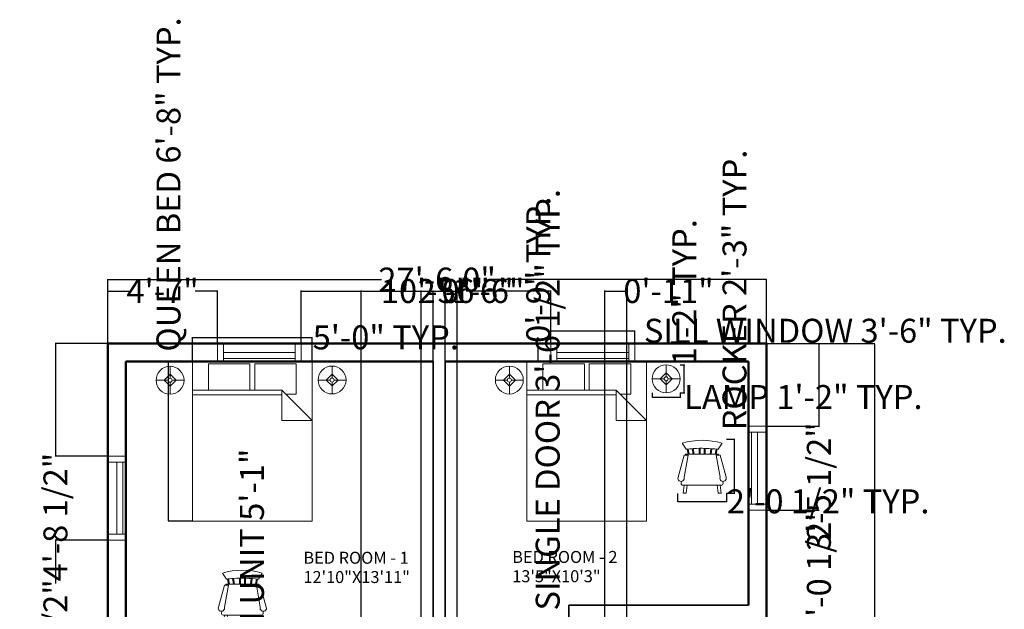
# Model space of a CAD drawing. Units: inches. Extents: x -52 to 472, y -40 to 644.
# Tile 6 of 6: x -21 to 472, y 349 to 644. Entities that reach past the tile are written whole.
import ezdxf

# ---------------------------------------------------------------- set-up
doc = ezdxf.new("R2010")
doc.units = ezdxf.units.IN
doc.header["$MEASUREMENT"] = 0
for name, color, linetype, lineweight in [('A-ANNO-DIMS', 7, 'Continuous', 13), ('A-ANNO-TEXT', 7, 'Continuous', 18), ('E-LIGHT', 30, 'Continuous', 13), ('FURNITURE', 6, 'Continuous', 13), ('INNER WALL', 1, 'Continuous', 35), ('OUTER WALL', 1, 'Continuous', 50), ('WINDOWS', 4, 'Continuous', 20)]:
    doc.layers.add(name, color=color, linetype=linetype, lineweight=lineweight)
doc.styles.get("Standard").update_dxf_attribs({"font": 'arial.ttf'})
doc.dimstyles.get("Standard").update_dxf_attribs({"dimtxt": 12, "dimasz": 0.18, "dimexe": 0.18, "dimexo": 0.0625, "dimgap": 0.09, "dimtad": 0, "dimdec": 1, "dimzin": 0, "dimdsep": 46, "dimlunit": 3, "dimtxsty": 'Standard', "dimcen": 0.09, "dimadec": 0, "dimazin": 0, "dimtfac": 1, "dimtdec": 1, "dimtofl": 0, "dimtmove": 0, "dimatfit": 3, "dimfxl": 1, "dimtolj": 1, "dimtzin": 0, "dimarcsym": 0})

# ---------------------------------------------------------------- blocks, each defined once
blk = doc.blocks.new('*D1')
at = {"layer": 'A-ANNO-DIMS', "color": 0, "lineweight": -2, "transparency": 16777216}
for p, q in [((23.13, 482.39), (23.13, 514.42)), ((23.31, 514.24), (160.34, 514.24)), ((352.95, 514.24), (215.93, 514.24)), ((353.13, 482.39), (353.13, 514.42))]:
    blk.add_line(p, q, dxfattribs=at)
at = {"layer": 'A-ANNO-DIMS', "color": 0, "transparency": 16777216}
for points in [[(23.31, 514.27), (23.31, 514.21), (23.13, 514.24)], [(352.95, 514.27), (352.95, 514.21), (353.13, 514.24)]]:
    blk.add_solid(points, dxfattribs=at)
at = {"layer": 'Defpoints', "color": 0, "transparency": 16777216}
for p in [(353.13, 514.24), (23.13, 482.33), (353.13, 482.33)]:
    blk.add_point(p, dxfattribs=at)
at = {"layer": 'A-ANNO-DIMS', "color": 0, "transparency": 16777216, "insert": (188.13, 514.24), "char_height": 12, "attachment_point": 5}
blk.add_mtext('\\A1;27\'-6.0"', dxfattribs=at)
blk = doc.blocks.new('*D2')
at = {"layer": 'A-ANNO-DIMS', "color": 0, "lineweight": -2, "transparency": 16777216}
for p, q in [((353.19, 482.33), (407.42, 482.33)), ((407.24, 482.15), (407.24, 275.68)), ((407.24, 4.51), (407.24, 210.98)), ((353.19, 4.33), (407.42, 4.33))]:
    blk.add_line(p, q, dxfattribs=at)
at = {"layer": 'A-ANNO-DIMS', "color": 0, "transparency": 16777216}
for points in [[(407.21, 482.15), (407.27, 482.15), (407.24, 482.33)], [(407.21, 4.51), (407.27, 4.51), (407.24, 4.33)]]:
    blk.add_solid(points, dxfattribs=at)
at = {"layer": 'Defpoints', "color": 0, "transparency": 16777216}
for p in [(353.13, 482.33), (353.13, 4.33), (407.24, 4.33)]:
    blk.add_point(p, dxfattribs=at)
at = {"layer": 'A-ANNO-DIMS', "color": 0, "transparency": 16777216, "insert": (407.24, 243.33), "char_height": 12, "attachment_point": 5, "rotation": 90}
blk.add_mtext('\\A1;39\'-10.0"', dxfattribs=at)
blk = doc.blocks.new('Chair - Rocking')
for p, q in [((-8, -4.5), (-10, -1.5)), ((-7.5, -4.5), (-7, -7)), ((-6.5, -7), (-7.02225, -4.43)), ((-4.5, -7), (-4.96674, -4.19951)), ((-4, -7), (-4.40532, -4.16272)), ((-1.5, -4.05012), (-1.5, -7)), ((-1, -7), (-1, -4.05012)), ((1, -7), (1, -4.04655)), ((1.5, -4.05012), (1.5, -7)), ((4, -7), (4.40187, -4.18694)), ((4.5, -7), (4.96761, -4.19437)), ((6.5, -7), (7, -4.4057)), ((7.5, -4.5), (7, -7)), ((8, -4.5), (10, -1.5)), ((-9, -7.5), (-12, -18.49999)), ((-7, -7.5), (-9, -7.5)), ((-9, -18.49999), (-7, -7.5)), ((-8.23428, -6.99939), (-8.3093, -7.47958)), ((-8.23041, -7), (8.23915, -7)), ((7, -7.5), (9, -7.5)), ((9, -18.49999), (7, -7.5)), ((8.31071, -7.48854), (8.23449, -7.00073)), ((9, -7.5), (12, -18.49999)), ((-10.36644, -20.64523), (-10.5, -21.49999)), ((-9, -22.49999), (-9.5, -26.49999)), ((0, -22.49999), (-9.5, -22.49999)), ((-8, -26.49999), (-7.5, -22.49999)), ((0, -22.49999), (9.5, -22.49999)), ((8, -26.49999), (7.5, -22.49999)), ((9, -22.49999), (9.5, -26.49999)), ((10.5, -21.49999), (10.3575, -20.58798)), ((-9.5, -26.49999), (-8, -26.49999)), ((9.5, -26.49999), (8, -26.49999))]:
    blk.add_line(p, q)
for centre, radius, start, end in [((0, -34.08333), 34.08333, 72.93847, 107.0615), ((0, -68.25004), 64.25, 93.92211, 97.15267), ((0, -68.25004), 64.25, 82.84733, 93.92211), ((-10.5, -18.99999), 1.58114, 161.5651, 18.43495), ((10.5, -18.99999), 1.58114, 161.5651, 18.43495), ((-9.5, -21.49999), 1, 180, 270), ((9.5, -21.49999), 1, 270, 0)]:
    blk.add_arc(centre, radius, start, end)
blk = doc.blocks.new('Bed - Queen')
for p, q in [((0, -80.00003), (0, 0)), ((0, 0), (59.99999, 0)), ((59.99999, 0), (59.99999, -80.00003)), ((7.99999, -1.2), (28.79998, -1.2)), ((7.99999, -14.4), (7.99999, -1.2)), ((28.79998, -1.2), (28.79998, -14.4)), ((31.19999, -1.2), (51.99999, -1.2)), ((31.19999, -14.4), (31.19999, -1.2)), ((51.99999, -1.2), (51.99999, -16.4)), ((0, -14.4), (44.8, -14.4)), ((59.99999, -29.6), (44.8, -14.4)), ((44.8, -14.4), (44.8, -29.6)), ((44.8, -16.8), (0, -16.8)), ((51.99999, -16.4), (46.79936, -16.4)), ((44.8, -29.6), (59.99999, -29.6)), ((59.99999, -80.00003), (0, -80.00003))]:
    blk.add_line(p, q)
blk = doc.blocks.new('Lamp - Table')
for p, q in [((0, 7), (0, 1)), ((-1, 0), (-7, 0)), ((0, 3), (-3, 0)), ((-3, 0), (0, -3)), ((3, 0), (0, 3)), ((0, -3), (3, 0)), ((1, 0), (7, 0)), ((0, -1), (0, -7))]:
    blk.add_line(p, q)
for radius in [7, 1]:
    blk.add_circle((0, 0), radius)
blk = doc.blocks.new('WIN-36IN')
for p, q in [((9, 42), (0, 42)), ((9, 39), (0, 39)), ((4.5, 3), (4.5, 39)), ((7.5, 3), (7.5, 39)), ((0, 3), (9, 3)), ((0, 0), (9, 0))]:
    blk.add_line(p, q)
blk = doc.blocks.new('WIN-36IN-SILL')
for p, q in [((0, 9), (0, 0)), ((3, 9), (3, 0)), ((39, 0), (39, 9)), ((42, 0), (42, 9)), ((3, 4.5), (39, 4.5)), ((3, 1.5), (39, 1.5)), ((3, 0), (39, 0))]:
    blk.add_line(p, q)
blk = doc.blocks.new('*D24')
at = {"layer": 'A-ANNO-DIMS', "color": 0, "lineweight": -2, "transparency": 16777216}
for p, q in [((295.84, 457.52), (295.84, 455.3)), ((296.02, 455.48), (309.66, 455.48)), ((309.84, 457.52), (309.84, 455.3)), ((309.84, 455.48), (310.02, 455.48))]:
    blk.add_line(p, q, dxfattribs=at)
at = {"layer": 'A-ANNO-DIMS', "color": 0, "transparency": 16777216}
for points in [[(296.02, 455.51), (296.02, 455.45), (295.84, 455.48)], [(309.66, 455.51), (309.66, 455.45), (309.84, 455.48)]]:
    blk.add_solid(points, dxfattribs=at)
at = {"layer": 'Defpoints', "color": 0, "transparency": 16777216}
for p in [(295.84, 457.58), (309.84, 457.58), (309.84, 455.48)]:
    blk.add_point(p, dxfattribs=at)
at = {"layer": 'A-ANNO-DIMS', "color": 0, "transparency": 16777216, "insert": (371.57, 455.48), "char_height": 12, "attachment_point": 5}
blk.add_mtext('\\A1;LAMP 1\'-2" TYP.', dxfattribs=at)
blk = doc.blocks.new('*D25')
at = {"layer": 'A-ANNO-DIMS', "color": 0, "lineweight": -2, "transparency": 16777216}
for p, q in [((309.9, 471.58), (312.12, 471.58)), ((311.94, 471.58), (311.94, 471.76)), ((311.94, 457.76), (311.94, 471.4)), ((309.9, 457.58), (312.12, 457.58))]:
    blk.add_line(p, q, dxfattribs=at)
at = {"layer": 'A-ANNO-DIMS', "color": 0, "transparency": 16777216}
for points in [[(311.91, 471.4), (311.97, 471.4), (311.94, 471.58)], [(311.91, 457.76), (311.97, 457.76), (311.94, 457.58)]]:
    blk.add_solid(points, dxfattribs=at)
at = {"layer": 'Defpoints', "color": 0, "transparency": 16777216}
for p in [(309.84, 471.58), (311.94, 471.58), (309.84, 457.58)]:
    blk.add_point(p, dxfattribs=at)
at = {"layer": 'A-ANNO-DIMS', "color": 0, "transparency": 16777216, "insert": (311.94, 507.86), "char_height": 12, "attachment_point": 5, "rotation": 90}
blk.add_mtext('\\A1;1\'-2" TYP.', dxfattribs=at)
blk = doc.blocks.new('*D28')
at = {"layer": 'A-ANNO-DIMS', "color": 0, "lineweight": -2, "transparency": 16777216}
for p, q in [((333.1, 434.31), (337.26, 434.31)), ((337.08, 434.31), (337.08, 434.49)), ((337.08, 407.49), (337.08, 434.13)), ((333.1, 407.31), (337.26, 407.31))]:
    blk.add_line(p, q, dxfattribs=at)
at = {"layer": 'A-ANNO-DIMS', "color": 0, "transparency": 16777216}
for points in [[(337.05, 434.13), (337.11, 434.13), (337.08, 434.31)], [(337.05, 407.49), (337.11, 407.49), (337.08, 407.31)]]:
    blk.add_solid(points, dxfattribs=at)
at = {"layer": 'Defpoints', "color": 0, "transparency": 16777216}
for p in [(333.03, 434.31), (337.08, 434.31), (333.03, 407.31)]:
    blk.add_point(p, dxfattribs=at)
at = {"layer": 'A-ANNO-DIMS', "color": 0, "transparency": 16777216, "insert": (337.08, 509.03), "char_height": 12, "attachment_point": 5, "rotation": 90}
blk.add_mtext('\\A1;ROCKER 2\'-3" TYP.', dxfattribs=at)
blk = doc.blocks.new('*D29')
at = {"layer": 'A-ANNO-DIMS', "color": 0, "lineweight": -2, "transparency": 16777216}
for p, q in [((308.6, 407.25), (308.6, 403.08)), ((333.03, 407.25), (333.03, 403.08)), ((308.78, 403.26), (332.85, 403.26)), ((333.03, 403.26), (333.21, 403.26))]:
    blk.add_line(p, q, dxfattribs=at)
at = {"layer": 'A-ANNO-DIMS', "color": 0, "transparency": 16777216}
for points in [[(308.78, 403.29), (308.78, 403.23), (308.6, 403.26)], [(332.85, 403.29), (332.85, 403.23), (333.03, 403.26)]]:
    blk.add_solid(points, dxfattribs=at)
at = {"layer": 'Defpoints', "color": 0, "transparency": 16777216}
for p in [(308.6, 407.31), (333.03, 407.31), (333.03, 403.26)]:
    blk.add_point(p, dxfattribs=at)
at = {"layer": 'A-ANNO-DIMS', "color": 0, "transparency": 16777216, "insert": (383.96, 403.26), "char_height": 12, "attachment_point": 5}
blk.add_mtext('\\A1;2\'-0 1/2" TYP.', dxfattribs=at)
blk = doc.blocks.new('*D30')
at = {"layer": 'A-ANNO-DIMS', "color": 0, "lineweight": -2, "transparency": 16777216}
for p, q in [((53.57, 473.33), (53.57, 473.51)), ((65.5, 473.33), (53.39, 473.33)), ((53.57, 393.51), (53.57, 473.15)), ((65.5, 393.33), (53.39, 393.33))]:
    blk.add_line(p, q, dxfattribs=at)
at = {"layer": 'A-ANNO-DIMS', "color": 0, "transparency": 16777216}
for points in [[(53.54, 473.15), (53.6, 473.15), (53.57, 473.33)], [(53.54, 393.51), (53.6, 393.51), (53.57, 393.33)]]:
    blk.add_solid(points, dxfattribs=at)
at = {"layer": 'Defpoints', "color": 0, "transparency": 16777216}
for p in [(53.57, 473.33), (65.57, 473.33), (65.57, 393.33)]:
    blk.add_point(p, dxfattribs=at)
at = {"layer": 'A-ANNO-DIMS', "color": 0, "transparency": 16777216, "insert": (53.57, 561.86), "char_height": 12, "attachment_point": 5, "rotation": 90}
blk.add_mtext('\\A1;QUEEN BED 6\'-8" TYP.', dxfattribs=at)
blk = doc.blocks.new('*D31')
at = {"layer": 'A-ANNO-DIMS', "color": 0, "lineweight": -2, "transparency": 16777216}
for p, q in [((65.57, 473.39), (65.57, 485.51)), ((65.75, 485.33), (125.39, 485.33)), ((125.57, 473.39), (125.57, 485.51)), ((125.57, 485.33), (125.75, 485.33))]:
    blk.add_line(p, q, dxfattribs=at)
at = {"layer": 'A-ANNO-DIMS', "color": 0, "transparency": 16777216}
for points in [[(65.75, 485.36), (65.75, 485.3), (65.57, 485.33)], [(125.39, 485.36), (125.39, 485.3), (125.57, 485.33)]]:
    blk.add_solid(points, dxfattribs=at)
at = {"layer": 'Defpoints', "color": 0, "transparency": 16777216}
for p in [(125.57, 485.33), (65.57, 473.33), (125.57, 473.33)]:
    blk.add_point(p, dxfattribs=at)
at = {"layer": 'A-ANNO-DIMS', "color": 0, "transparency": 16777216, "insert": (162.41, 485.33), "char_height": 12, "attachment_point": 5}
blk.add_mtext('\\A1;5\'-0" TYP.', dxfattribs=at)
blk = doc.blocks.new('*D36')
at = {"layer": 'A-ANNO-DIMS', "color": 0, "lineweight": -2, "transparency": 16777216}
for p, q in [((245.07, 482.39), (245.07, 488.81)), ((245.25, 488.63), (286.89, 488.63)), ((287.07, 482.39), (287.07, 488.81)), ((287.07, 488.63), (287.25, 488.63))]:
    blk.add_line(p, q, dxfattribs=at)
at = {"layer": 'A-ANNO-DIMS', "color": 0, "transparency": 16777216}
for points in [[(245.25, 488.66), (245.25, 488.6), (245.07, 488.63)], [(286.89, 488.66), (286.89, 488.6), (287.07, 488.63)]]:
    blk.add_solid(points, dxfattribs=at)
at = {"layer": 'Defpoints', "color": 0, "transparency": 16777216}
for p in [(287.07, 488.63), (245.07, 482.33), (287.07, 482.33)]:
    blk.add_point(p, dxfattribs=at)
at = {"layer": 'A-ANNO-DIMS', "color": 0, "transparency": 16777216, "insert": (382.56, 488.63), "char_height": 12, "attachment_point": 5}
blk.add_mtext('\\A1;SILL WINDOW 3\'-6" TYP.', dxfattribs=at)
blk = doc.blocks.new('*D37')
at = {"layer": 'A-ANNO-DIMS', "color": 0, "lineweight": -2, "transparency": 16777216}
for p, q in [((245, 482.33), (238.59, 482.33)), ((238.77, 482.33), (238.77, 482.51)), ((238.77, 473.51), (238.77, 482.15)), ((245, 473.33), (238.59, 473.33))]:
    blk.add_line(p, q, dxfattribs=at)
at = {"layer": 'A-ANNO-DIMS', "color": 0, "transparency": 16777216}
for points in [[(238.74, 482.15), (238.8, 482.15), (238.77, 482.33)], [(238.74, 473.51), (238.8, 473.51), (238.77, 473.33)]]:
    blk.add_solid(points, dxfattribs=at)
at = {"layer": 'Defpoints', "color": 0, "transparency": 16777216}
for p in [(238.77, 482.33), (245.07, 482.33), (245.07, 473.33)]:
    blk.add_point(p, dxfattribs=at)
at = {"layer": 'A-ANNO-DIMS', "color": 0, "transparency": 16777216, "insert": (238.77, 519.17), "char_height": 12, "attachment_point": 5, "rotation": 90}
blk.add_mtext('\\A1;0\'-9" TYP.', dxfattribs=at)
blk = doc.blocks.new('*D50')
at = {"layer": 'A-ANNO-DIMS', "color": 0, "lineweight": -2, "transparency": 16777216}
for p, q in [((237.19, 342.75), (243.68, 342.75)), ((243.5, 342.75), (243.5, 342.93)), ((243.5, 300.51), (243.5, 342.57)), ((237.19, 300.33), (243.68, 300.33))]:
    blk.add_line(p, q, dxfattribs=at)
at = {"layer": 'A-ANNO-DIMS', "color": 0, "transparency": 16777216}
for points in [[(243.47, 342.57), (243.53, 342.57), (243.5, 342.75)], [(243.47, 300.51), (243.53, 300.51), (243.5, 300.33)]]:
    blk.add_solid(points, dxfattribs=at)
at = {"layer": 'Defpoints', "color": 0, "transparency": 16777216}
for p in [(237.13, 342.75), (243.5, 342.75), (237.13, 300.33)]:
    blk.add_point(p, dxfattribs=at)
at = {"layer": 'A-ANNO-DIMS', "color": 0, "transparency": 16777216, "insert": (243.5, 454.09), "char_height": 12, "attachment_point": 5, "rotation": 90}
blk.add_mtext('\\A1;SINGLE DOOR 3\'-6 1/2" TYP.', dxfattribs=at)
blk = doc.blocks.new('*D62')
at = {"layer": 'A-ANNO-DIMS', "color": 0, "lineweight": -2, "transparency": 16777216}
for p, q in [((86.27, 277.33), (95.54, 277.33)), ((95.36, 277.33), (95.36, 277.51)), ((95.36, 216.51), (95.36, 277.15)), ((86.27, 216.33), (95.54, 216.33))]:
    blk.add_line(p, q, dxfattribs=at)
at = {"layer": 'A-ANNO-DIMS', "color": 0, "transparency": 16777216}
for points in [[(95.33, 277.15), (95.39, 277.15), (95.36, 277.33)], [(95.33, 216.51), (95.39, 216.51), (95.36, 216.33)]]:
    blk.add_solid(points, dxfattribs=at)
at = {"layer": 'Defpoints', "color": 0, "transparency": 16777216}
for p in [(86.21, 277.33), (95.36, 277.33), (86.21, 216.33)]:
    blk.add_point(p, dxfattribs=at)
at = {"layer": 'A-ANNO-DIMS', "color": 0, "transparency": 16777216, "insert": (95.36, 354.29), "char_height": 12, "attachment_point": 5, "rotation": 90}
blk.add_mtext('\\A1;KITCHEN UNIT 5\'-1"', dxfattribs=at)
blk = doc.blocks.new('*D64')
at = {"layer": 'A-ANNO-DIMS', "color": 0, "lineweight": -2, "transparency": 16777216}
for p, q in [((23.13, 482.39), (23.13, 508.71)), ((23.31, 508.53), (34.32, 508.53)), ((77.89, 508.53), (66.88, 508.53)), ((78.07, 482.39), (78.07, 508.71))]:
    blk.add_line(p, q, dxfattribs=at)
at = {"layer": 'A-ANNO-DIMS', "color": 0, "transparency": 16777216}
for points in [[(23.31, 508.56), (23.31, 508.5), (23.13, 508.53)], [(77.89, 508.56), (77.89, 508.5), (78.07, 508.53)]]:
    blk.add_solid(points, dxfattribs=at)
at = {"layer": 'Defpoints', "color": 0, "transparency": 16777216}
for p in [(78.07, 508.53), (23.13, 482.33), (78.07, 482.33)]:
    blk.add_point(p, dxfattribs=at)
at = {"layer": 'A-ANNO-DIMS', "color": 0, "transparency": 16777216, "insert": (50.6, 508.53), "char_height": 12, "attachment_point": 5}
blk.add_mtext('\\A1;4\'-7"', dxfattribs=at)
blk = doc.blocks.new('*D65')
at = {"layer": 'A-ANNO-DIMS', "color": 0, "lineweight": -2, "transparency": 16777216}
for p, q in [((120.07, 482.39), (120.07, 508.71)), ((120.25, 508.53), (162.43, 508.53)), ((244.89, 508.53), (202.7, 508.53)), ((245.07, 482.39), (245.07, 508.71))]:
    blk.add_line(p, q, dxfattribs=at)
at = {"layer": 'A-ANNO-DIMS', "color": 0, "transparency": 16777216}
for points in [[(120.25, 508.56), (120.25, 508.5), (120.07, 508.53)], [(244.89, 508.56), (244.89, 508.5), (245.07, 508.53)]]:
    blk.add_solid(points, dxfattribs=at)
at = {"layer": 'Defpoints', "color": 0, "transparency": 16777216}
for p in [(245.07, 508.53), (120.07, 482.33), (245.07, 482.33)]:
    blk.add_point(p, dxfattribs=at)
at = {"layer": 'A-ANNO-DIMS', "color": 0, "transparency": 16777216, "insert": (182.57, 508.53), "char_height": 12, "attachment_point": 5}
blk.add_mtext('\\A1;10\'-5"', dxfattribs=at)
blk = doc.blocks.new('*D66')
at = {"layer": 'A-ANNO-DIMS', "color": 0, "lineweight": -2, "transparency": 16777216}
for p, q in [((23.07, 482.33), (-3.25, 482.33)), ((-3.07, 482.15), (-3.07, 425.99)), ((23.07, 425.81), (-3.25, 425.81)), ((-3.07, 425.81), (-3.07, 425.63))]:
    blk.add_line(p, q, dxfattribs=at)
at = {"layer": 'A-ANNO-DIMS', "color": 0, "transparency": 16777216}
for points in [[(-3.1, 482.15), (-3.04, 482.15), (-3.07, 482.33)], [(-3.1, 425.99), (-3.04, 425.99), (-3.07, 425.81)]]:
    blk.add_solid(points, dxfattribs=at)
at = {"layer": 'Defpoints', "color": 0, "transparency": 16777216}
for p in [(23.13, 482.33), (-3.07, 425.81), (23.13, 425.81)]:
    blk.add_point(p, dxfattribs=at)
at = {"layer": 'A-ANNO-DIMS', "color": 0, "transparency": 16777216, "insert": (-3.07, 395.37), "char_height": 12, "attachment_point": 5, "rotation": 90}
blk.add_mtext('\\A1;4\'-8 1/2"', dxfattribs=at)
blk = doc.blocks.new('*D67')
at = {"layer": 'A-ANNO-DIMS', "color": 0, "lineweight": -2, "transparency": 16777216}
for p, q in [((23.07, 383.81), (-3.25, 383.81)), ((-3.07, 383.63), (-3.07, 362.09)), ((-3.07, 280.49), (-3.07, 302.03)), ((23.07, 280.31), (-3.25, 280.31))]:
    blk.add_line(p, q, dxfattribs=at)
at = {"layer": 'A-ANNO-DIMS', "color": 0, "transparency": 16777216}
for points in [[(-3.1, 383.63), (-3.04, 383.63), (-3.07, 383.81)], [(-3.1, 280.49), (-3.04, 280.49), (-3.07, 280.31)]]:
    blk.add_solid(points, dxfattribs=at)
at = {"layer": 'Defpoints', "color": 0, "transparency": 16777216}
for p in [(23.13, 383.81), (-3.07, 280.31), (23.13, 280.31)]:
    blk.add_point(p, dxfattribs=at)
at = {"layer": 'A-ANNO-DIMS', "color": 0, "transparency": 16777216, "insert": (-3.07, 332.06), "char_height": 12, "attachment_point": 5, "rotation": 90}
blk.add_mtext('\\A1;8\'-7 1/2"', dxfattribs=at)
blk = doc.blocks.new('*D69')
at = {"layer": 'A-ANNO-DIMS', "color": 0, "lineweight": -2, "transparency": 16777216}
for p, q in [((353.19, 482.33), (379.51, 482.33)), ((379.33, 482.15), (379.33, 440.99)), ((353.19, 440.81), (379.51, 440.81)), ((379.33, 440.81), (379.33, 440.63))]:
    blk.add_line(p, q, dxfattribs=at)
at = {"layer": 'A-ANNO-DIMS', "color": 0, "transparency": 16777216}
for points in [[(379.3, 482.15), (379.36, 482.15), (379.33, 482.33)], [(379.3, 440.99), (379.36, 440.99), (379.33, 440.81)]]:
    blk.add_solid(points, dxfattribs=at)
at = {"layer": 'Defpoints', "color": 0, "transparency": 16777216}
for p in [(353.13, 482.33), (353.13, 440.81), (379.33, 440.81)]:
    blk.add_point(p, dxfattribs=at)
at = {"layer": 'A-ANNO-DIMS', "color": 0, "transparency": 16777216, "insert": (379.33, 410.61), "char_height": 12, "attachment_point": 5, "rotation": 90}
blk.add_mtext('\\A1;3\'-5 1/2"', dxfattribs=at)
blk = doc.blocks.new('*D70')
at = {"layer": 'A-ANNO-DIMS', "color": 0, "lineweight": -2, "transparency": 16777216}
for p, q in [((353.194987, 398.808713), (379.512487, 398.808713)), ((379.332487, 398.988713), (379.332487, 399.168713)), ((353.194987, 338.308713), (379.512487, 338.308713)), ((379.332487, 338.128713), (379.332487, 337.948713))]:
    blk.add_line(p, q, dxfattribs=at)
at = {"layer": 'A-ANNO-DIMS', "color": 0, "transparency": 16777216}
for points in [[(379.302487, 398.988713), (379.362487, 398.988713), (379.332487, 398.808713)], [(379.302487, 338.128713), (379.362487, 338.128713), (379.332487, 338.308713)]]:
    blk.add_solid(points, dxfattribs=at)
at = {"layer": 'Defpoints', "color": 0, "transparency": 16777216}
for p in [(353.132487, 398.808713), (353.132487, 338.308713), (379.332487, 338.308713)]:
    blk.add_point(p, dxfattribs=at)
at = {"layer": 'A-ANNO-DIMS', "color": 0, "transparency": 16777216, "insert": (379.332487, 368.558713), "char_height": 12, "attachment_point": 5, "rotation": 90}
blk.add_mtext('\\A1;5\'-0 1/2"', dxfattribs=at)
blk = doc.blocks.new('*D77')
at = {"layer": 'A-ANNO-DIMS', "color": 0, "lineweight": -2, "transparency": 16777216}
for p, q in [((186.13, 473.39), (186.13, 508.71)), ((186.31, 508.53), (191.95, 508.53)), ((192.13, 473.39), (192.13, 508.71)), ((192.13, 508.53), (192.31, 508.53))]:
    blk.add_line(p, q, dxfattribs=at)
at = {"layer": 'A-ANNO-DIMS', "color": 0, "transparency": 16777216}
for points in [[(186.31, 508.56), (186.31, 508.5), (186.13, 508.53)], [(191.95, 508.56), (191.95, 508.5), (192.13, 508.53)]]:
    blk.add_solid(points, dxfattribs=at)
at = {"layer": 'Defpoints', "color": 0, "transparency": 16777216}
for p in [(192.13, 508.53), (186.13, 473.33), (192.13, 473.33)]:
    blk.add_point(p, dxfattribs=at)
at = {"layer": 'A-ANNO-DIMS', "color": 0, "transparency": 16777216, "insert": (208.35, 508.53), "char_height": 12, "attachment_point": 5}
blk.add_mtext('\\A1;0\'-6"', dxfattribs=at)
blk = doc.blocks.new('*D79')
at = {"layer": 'A-ANNO-DIMS', "color": 0, "lineweight": -2, "transparency": 16777216}
for p, q in [((272.13, 206.39), (272.13, 508.71)), ((272.31, 508.53), (282.95, 508.53)), ((283.13, 206.39), (283.13, 508.71)), ((283.13, 508.53), (283.31, 508.53))]:
    blk.add_line(p, q, dxfattribs=at)
at = {"layer": 'A-ANNO-DIMS', "color": 0, "transparency": 16777216}
for points in [[(272.31, 508.56), (272.31, 508.5), (272.13, 508.53)], [(282.95, 508.56), (282.95, 508.5), (283.13, 508.53)]]:
    blk.add_solid(points, dxfattribs=at)
at = {"layer": 'Defpoints', "color": 0, "transparency": 16777216}
for p in [(283.13, 508.53), (272.13, 206.33), (283.13, 206.33)]:
    blk.add_point(p, dxfattribs=at)
at = {"layer": 'A-ANNO-DIMS', "color": 0, "transparency": 16777216, "insert": (304.01, 508.53), "char_height": 12, "attachment_point": 5}
blk.add_mtext('\\A1;0\'-11"', dxfattribs=at)
blk = doc.blocks.new('*D80')
at = {"layer": 'A-ANNO-DIMS', "color": 0, "lineweight": -2, "transparency": 16777216}
for p, q in [((150.13, 306.39), (150.13, 508.71)), ((150.31, 508.53), (179.95, 508.53)), ((180.13, 306.39), (180.13, 508.71)), ((180.13, 508.53), (180.31, 508.53))]:
    blk.add_line(p, q, dxfattribs=at)
at = {"layer": 'A-ANNO-DIMS', "color": 0, "transparency": 16777216}
for points in [[(150.31, 508.56), (150.31, 508.5), (150.13, 508.53)], [(179.95, 508.56), (179.95, 508.5), (180.13, 508.53)]]:
    blk.add_solid(points, dxfattribs=at)
at = {"layer": 'Defpoints', "color": 0, "transparency": 16777216}
for p in [(180.13, 508.53), (150.13, 306.33), (180.13, 306.33)]:
    blk.add_point(p, dxfattribs=at)
at = {"layer": 'A-ANNO-DIMS', "color": 0, "transparency": 16777216, "insert": (196.45, 508.53), "char_height": 12, "attachment_point": 5}
blk.add_mtext('\\A1;2\'-6"', dxfattribs=at)
blk = doc.blocks.new('*D81')
at = {"layer": 'A-ANNO-DIMS', "color": 0, "lineweight": -2, "transparency": 16777216}
for p, q in [((180.13, 306.39), (180.13, 508.71)), ((180.31, 508.53), (197.95, 508.53)), ((198.13, 306.39), (198.13, 508.71)), ((198.13, 508.53), (198.31, 508.53))]:
    blk.add_line(p, q, dxfattribs=at)
at = {"layer": 'A-ANNO-DIMS', "color": 0, "transparency": 16777216}
for points in [[(180.31, 508.56), (180.31, 508.5), (180.13, 508.53)], [(197.95, 508.56), (197.95, 508.5), (198.13, 508.53)]]:
    blk.add_solid(points, dxfattribs=at)
at = {"layer": 'Defpoints', "color": 0, "transparency": 16777216}
for p in [(198.13, 508.53), (180.13, 306.33), (198.13, 306.33)]:
    blk.add_point(p, dxfattribs=at)
at = {"layer": 'A-ANNO-DIMS', "color": 0, "transparency": 16777216, "insert": (213.79, 508.53), "char_height": 12, "attachment_point": 5}
blk.add_mtext('\\A1;1\'-6"', dxfattribs=at)

msp = doc.modelspace()

# ---------------------------------------------------------------- linework, layer by layer
at = {"layer": 'INNER WALL'}
for p, q in [((186.13, 473.33), (186.13, 306.33)), ((192.13, 473.33), (192.13, 306.33)), ((344.13, 351.33), (254.13, 351.33)), ((254.13, 341.33), (254.13, 351.33))]:
    msp.add_line(p, q, dxfattribs=at)
at = {"layer": 'OUTER WALL'}
for p, q in [((32.13, 473.33), (32.13, 306.33)), ((186.13, 473.33), (32.13, 473.33)), ((344.13, 473.33), (192.13, 473.33)), ((344.13, 351.33), (344.13, 473.33))]:
    msp.add_line(p, q, dxfattribs=at)
msp.add_lwpolyline([(208.13, 4.33), (353.13, 4.33), (353.13, 482.33), (23.13, 482.33), (23.13, 4.33), (136.13, 4.33)], dxfattribs=at)

# ---------------------------------------------------------------- block references
at = {"layer": 'E-LIGHT'}
for p in [(54.36, 463.87), (135.48, 463.99), (224.3, 463.96), (302.84, 464.58)]:
    msp.add_blockref('Lamp - Table', p, dxfattribs=at)
at = {"layer": 'FURNITURE'}
for name, p in [('Bed - Queen', (65.57, 473.33)), ('Bed - Queen', (233.07, 473.33)), ('Chair - Rocking', (320.82, 433.81)), ('Chair - Rocking', (90.57, 368.81))]:
    msp.add_blockref(name, p, dxfattribs=at)
at = {"layer": 'WINDOWS'}
for name, p in [('WIN-36IN-SILL', (78.07, 473.33)), ('WIN-36IN-SILL', (245.07, 473.33)), ('WIN-36IN', (23.13, 383.81))]:
    msp.add_blockref(name, p, dxfattribs=at)
at = {"layer": 'WINDOWS', "rotation": 180}
msp.add_blockref('WIN-36IN', (353.13, 440.81), dxfattribs=at)

# ---------------------------------------------------------------- texts
at = {"layer": 'A-ANNO-TEXT'}
for s, p in [('BED ROOM - 1', (121.15, 372.02)), ('BED ROOM - 2', (225.75, 372.42)), ('12\'10"X13\'11"', (121.15, 362.38)), ('13\'5"X10\'3"', (225.75, 362.78))]:
    msp.add_text(s, height=6, dxfattribs=at).set_placement(p)

# ---------------------------------------------------------------- dimensions: what is measured, and where the dimension line sits
at = {"layer": 'A-ANNO-DIMS'}
for base, p1, p2, text, picture, middle in [((53.57, 473.33), (65.57, 393.33), (65.57, 473.33), 'QUEEN BED <> TYP.', '*D30', (53.57, 561.86)), ((337.08, 434.31), (333.03, 407.31), (333.03, 434.31), 'ROCKER <> TYP.', '*D28', (337.08, 509.03)), ((243.5, 342.75), (237.13, 300.33), (237.13, 342.75), 'SINGLE DOOR <> TYP.', '*D50', (243.5, 454.09)), ((238.77, 482.33), (245.07, 473.33), (245.07, 482.33), '<> TYP.', '*D37', (238.77, 519.17)), ((311.94, 471.58), (309.84, 457.58), (309.84, 471.58), '<> TYP.', '*D25', (311.94, 507.86)), ((95.36, 277.33), (86.21, 216.33), (86.21, 277.33), 'KITCHEN UNIT <>', '*D62', (95.36, 354.29))]:
    dim = msp.add_linear_dim(base=base, p1=p1, p2=p2, angle=90, text=text, dimstyle='Standard', override={"dimdec": 1, "dimlfac": 1, "dimrnd": 0, "dimzin": 1, "dimdsep": 46, "dimlunit": 4, "dimfrac": 2}, dxfattribs=at)
    dim.commit()
    dim.dimension.update_dxf_attribs({"geometry": picture, "text_midpoint": middle})
for base, p1, p2, text, picture, middle in [((287.07, 488.63), (245.07, 482.33), (287.07, 482.33), 'SILL WINDOW <> TYP.', '*D36', (382.56, 488.63)), ((125.57, 485.33), (65.57, 473.33), (125.57, 473.33), '<> TYP.', '*D31', (162.41, 485.33)), ((309.84, 455.48), (295.84, 457.58), (309.84, 457.58), 'LAMP <> TYP.', '*D24', (371.57, 455.48)), ((333.03, 403.26), (308.6, 407.31), (333.03, 407.31), '<> TYP.', '*D29', (383.96, 403.26))]:
    dim = msp.add_linear_dim(base=base, p1=p1, p2=p2, text=text, dimstyle='Standard', override={"dimdec": 1, "dimlfac": 1, "dimrnd": 0, "dimzin": 1, "dimdsep": 46, "dimlunit": 4, "dimfrac": 2}, dxfattribs=at)
    dim.commit()
    dim.dimension.update_dxf_attribs({"geometry": picture, "text_midpoint": middle})
for base, p1, p2, override, picture, middle in [((353.13, 514.24), (23.13, 482.33), (353.13, 482.33), {"dimclrd": 0, "dimclre": 0, "dimclrt": 0}, '*D1', (188.13, 514.24)), ((78.07, 508.53), (23.13, 482.33), (78.07, 482.33), {"dimdec": 1, "dimlfac": 1, "dimrnd": 0, "dimzin": 1, "dimdsep": 46, "dimlunit": 4, "dimfrac": 2}, '*D64', (50.6, 508.53)), ((245.07, 508.53), (120.07, 482.33), (245.07, 482.33), {"dimdec": 1, "dimlfac": 1, "dimrnd": 0, "dimzin": 1, "dimdsep": 46, "dimlunit": 4, "dimfrac": 2}, '*D65', (182.57, 508.53)), ((180.13, 508.53), (150.13, 306.33), (180.13, 306.33), {"dimdec": 1, "dimlfac": 1, "dimrnd": 0, "dimzin": 1, "dimdsep": 46, "dimlunit": 4, "dimfrac": 2}, '*D80', (196.45, 508.53)), ((198.13, 508.53), (180.13, 306.33), (198.13, 306.33), {"dimdec": 1, "dimlfac": 1, "dimrnd": 0, "dimzin": 1, "dimdsep": 46, "dimlunit": 4, "dimfrac": 2}, '*D81', (213.79, 508.53)), ((192.13, 508.53), (186.13, 473.33), (192.13, 473.33), {"dimdec": 1, "dimlfac": 1, "dimrnd": 0, "dimzin": 1, "dimdsep": 46, "dimlunit": 4, "dimfrac": 2}, '*D77', (208.35, 508.53)), ((283.13, 508.53), (272.13, 206.33), (283.13, 206.33), {"dimdec": 1, "dimlfac": 1, "dimrnd": 0, "dimzin": 1, "dimdsep": 46, "dimlunit": 4, "dimfrac": 2}, '*D79', (304.01, 508.53))]:
    dim = msp.add_linear_dim(base=base, p1=p1, p2=p2, dimstyle='Standard', override=override, dxfattribs=at)
    dim.commit()
    dim.dimension.update_dxf_attribs({"geometry": picture, "text_midpoint": middle})
for base, p1, p2, override, picture, middle in [((-3.07, 425.81), (23.13, 482.33), (23.13, 425.81), {"dimdec": 1, "dimlfac": 1, "dimrnd": 0, "dimzin": 1, "dimdsep": 46, "dimlunit": 4, "dimfrac": 2}, '*D66', (-3.07, 395.37)), ((407.24, 4.33), (353.13, 482.33), (353.13, 4.33), {"dimclrd": 0, "dimclre": 0, "dimclrt": 0}, '*D2', (407.24, 243.33)), ((379.33, 440.81), (353.13, 482.33), (353.13, 440.81), {"dimdec": 1, "dimlfac": 1, "dimrnd": 0, "dimzin": 1, "dimdsep": 46, "dimlunit": 4, "dimfrac": 2}, '*D69', (379.33, 410.61)), ((379.33, 338.31), (353.13, 398.81), (353.13, 338.31), {"dimdec": 1, "dimlfac": 1, "dimrnd": 0, "dimzin": 1, "dimdsep": 46, "dimlunit": 4, "dimfrac": 2}, '*D70', (379.33, 368.56)), ((-3.07, 280.31), (23.13, 383.81), (23.13, 280.31), {"dimdec": 1, "dimlfac": 1, "dimrnd": 0, "dimzin": 1, "dimdsep": 46, "dimlunit": 4, "dimfrac": 2}, '*D67', (-3.07, 332.06))]:
    dim = msp.add_linear_dim(base=base, p1=p1, p2=p2, angle=90, dimstyle='Standard', override=override, dxfattribs=at)
    dim.commit()
    dim.dimension.update_dxf_attribs({"geometry": picture, "text_midpoint": middle})

doc.saveas('drawing.dxf')
